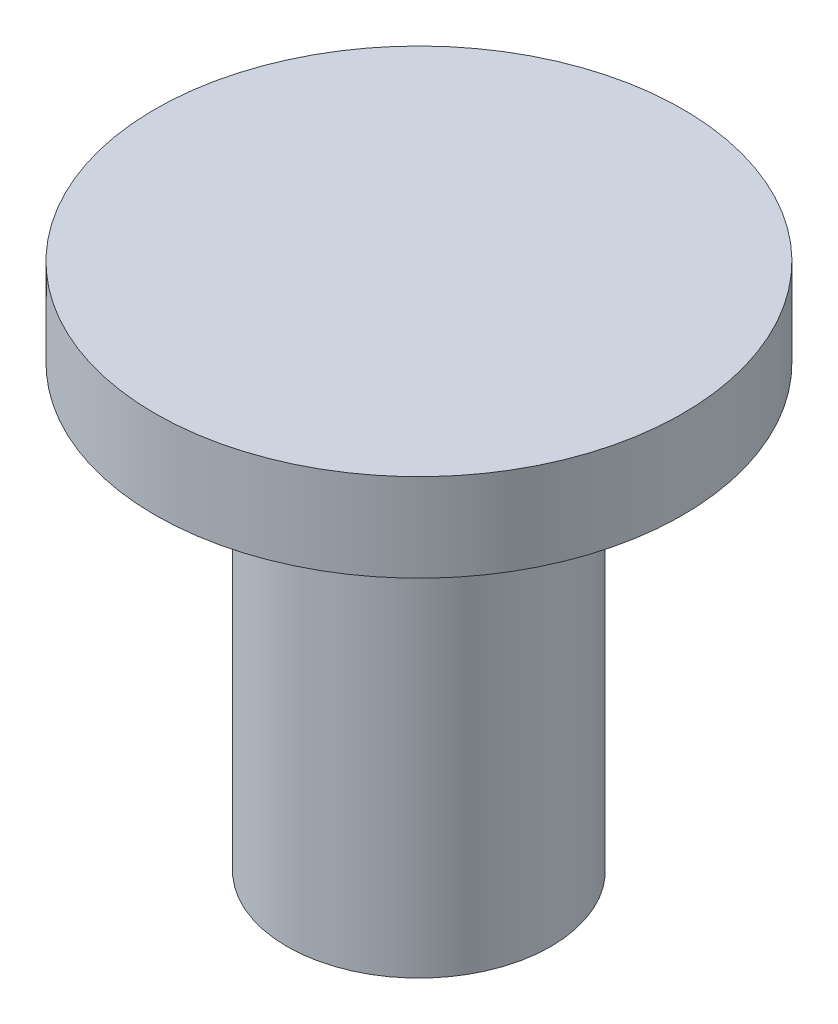
SolidWorks part; units mm, degrees
material "Plain Carbon Steel"
ref_plane "Front Plane" through (0, 0, 0) normal (0, 0, 1) x (1, 0, 0)
ref_plane "Top Plane" through (0, 0, 0) normal (0, 1, 0) x (1, 0, 0)
ref_plane "Right Plane" through (0, 0, 0) normal (1, 0, 0) x (0, 0, -1)
sketch "Shank Profile Ø6" plane through (0, 0, 0) normal (0, 1, 0) x (1, 0, 0)
  circle A0 centre (0, 0) radius 3
  dimension "D1" = 6
extrude "Shank Ø6x10" add sketch "Shank Profile Ø6" along normal blind 10
sketch "Head Profile Ø12" plane through (0, 10, 0) normal (0, 1, 0) x (1, 0, 0)
  circle A0 centre (0, 0) radius 6
  dimension "D1" = 12
extrude "Head Ø12x2" add sketch "Head Profile Ø12" along normal blind 2
